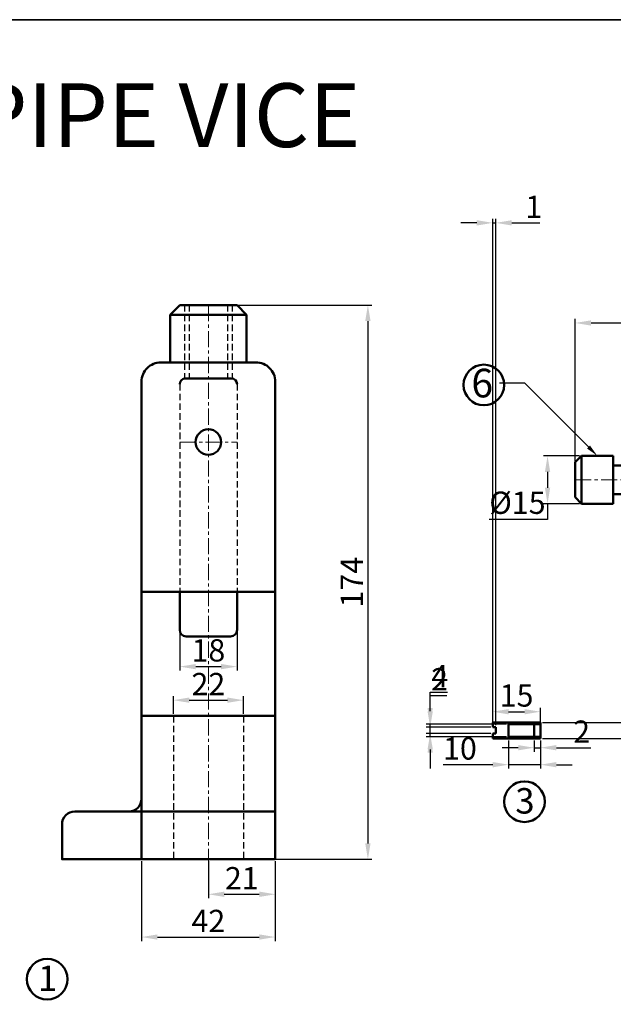
# Model space of a CAD drawing. Units: millimetres. Extents: x -39 to 854, y -107 to 478.
# Tile 3 of 4: x 309 to 496, y 169 to 478. Entities that reach past the tile are written whole.
import ezdxf
from ezdxf import colors
from ezdxf.entities.mleader import LeaderData, LeaderLine
from ezdxf.math import Vec2, Vec3

# ---------------------------------------------------------------- set-up
doc = ezdxf.new("R2010")
doc.units = ezdxf.units.MM
doc.header["$LTSCALE"] = 0.4
doc.linetypes.add('CENTER', pattern=[50.8, 31.75, -6.35, 6.35, -6.35])
doc.linetypes.add('DASHED', pattern=[19.05, 12.7, -6.35])
for name, color, linetype, lineweight in [('M-CNTR', 1, 'CENTER', 18), ('M-DIMS', 2, 'Continuous', 25), ('M-HIDN', 6, 'DASHED', 25), ('M-OUTL', 7, 'Continuous', 50), ('M-TEXT', 3, 'Continuous', 25), ('M-TTLB', 7, 'Continuous', 35)]:
    doc.layers.add(name, color=color, linetype=linetype, lineweight=lineweight)
doc.styles.get("Standard").update_dxf_attribs({"font": 'arial.ttf'})
doc.dimstyles.new('ISO-25', dxfattribs={"dimtxt": 7, "dimasz": 5, "dimexe": 1.25, "dimexo": 0.625, "dimtad": 1, "dimtoh": 1, "dimtxsty": 'Standard', "dimcen": 2.5, "dimadec": 0, "dimazin": 0, "dimtfac": 1, "dimtmove": 0, "dimatfit": 3, "dimfxl": 1, "dimarcsym": 0})

# ---------------------------------------------------------------- blocks, each defined once
blk = doc.blocks.new('*D41')
at = {"layer": 'Defpoints', "color": 0, "ltscale": 0.4, "transparency": 16777216}
for p in [(368.36, 388.19), (368.36, 214.19), (418.49, 214.19)]:
    blk.add_point(p, dxfattribs=at)
at = {"layer": 'M-DIMS', "color": 0, "lineweight": -2, "ltscale": 0.4, "transparency": 16777216}
for p, q in [((368.98, 388.19), (419.74, 388.19)), ((418.49, 383.19), (418.49, 219.19)), ((368.98, 214.19), (419.74, 214.19))]:
    blk.add_line(p, q, dxfattribs=at)
at = {"layer": 'M-DIMS', "color": 0, "ltscale": 0.4, "transparency": 16777216}
for points in [[(417.65, 383.19), (419.32, 383.19), (418.49, 388.19)], [(417.65, 219.19), (419.32, 219.19), (418.49, 214.19)]]:
    blk.add_solid(points, dxfattribs=at)
at = {"layer": 'M-DIMS', "color": 0, "ltscale": 0.4, "transparency": 16777216, "insert": (414.35, 301.19), "char_height": 7, "attachment_point": 5, "rotation": 90}
blk.add_mtext('174', dxfattribs=at)
blk = doc.blocks.new('*D42')
at = {"layer": 'Defpoints', "color": 0, "ltscale": 0.4, "transparency": 16777216}
for p in [(359.36, 292.19), (377.36, 292.19), (377.36, 274.68)]:
    blk.add_point(p, dxfattribs=at)
at = {"layer": 'M-DIMS', "color": 0, "lineweight": -2, "ltscale": 0.4, "transparency": 16777216}
for p, q in [((359.36, 291.56), (359.36, 273.43)), ((377.36, 291.56), (377.36, 273.43)), ((364.36, 274.68), (372.36, 274.68))]:
    blk.add_line(p, q, dxfattribs=at)
at = {"layer": 'M-DIMS', "color": 0, "ltscale": 0.4, "transparency": 16777216}
for points in [[(364.36, 275.51), (364.36, 273.85), (359.36, 274.68)], [(372.36, 275.51), (372.36, 273.85), (377.36, 274.68)]]:
    blk.add_solid(points, dxfattribs=at)
at = {"layer": 'M-DIMS', "color": 0, "ltscale": 0.4, "transparency": 16777216, "insert": (368.36, 278.88), "char_height": 7, "attachment_point": 5}
blk.add_mtext('18', dxfattribs=at)
blk = doc.blocks.new('*D43')
at = {"layer": 'Defpoints', "color": 0, "ltscale": 0.4, "transparency": 16777216}
for p in [(379.36, 264.15), (357.36, 259.19), (379.36, 259.19)]:
    blk.add_point(p, dxfattribs=at)
at = {"layer": 'M-DIMS', "color": 0, "lineweight": -2, "ltscale": 0.4, "transparency": 16777216}
for p, q in [((357.36, 259.81), (357.36, 265.4)), ((362.36, 264.15), (374.36, 264.15)), ((379.36, 259.81), (379.36, 265.4))]:
    blk.add_line(p, q, dxfattribs=at)
at = {"layer": 'M-DIMS', "color": 0, "ltscale": 0.4, "transparency": 16777216}
for points in [[(362.36, 264.98), (362.36, 263.32), (357.36, 264.15)], [(374.36, 264.98), (374.36, 263.32), (379.36, 264.15)]]:
    blk.add_solid(points, dxfattribs=at)
at = {"layer": 'M-DIMS', "color": 0, "ltscale": 0.4, "transparency": 16777216, "insert": (368.36, 268.29), "char_height": 7, "attachment_point": 5}
blk.add_mtext('22', dxfattribs=at)
blk = doc.blocks.new('*D44')
at = {"layer": 'Defpoints', "color": 0, "ltscale": 0.4, "transparency": 16777216}
for p in [(368.36, 214.19), (389.36, 214.19), (389.36, 203.2)]:
    blk.add_point(p, dxfattribs=at)
at = {"layer": 'M-DIMS', "color": 0, "lineweight": -2, "ltscale": 0.4, "transparency": 16777216}
for p, q in [((368.36, 213.56), (368.36, 201.95)), ((389.36, 213.56), (389.36, 201.95)), ((373.36, 203.2), (384.36, 203.2))]:
    blk.add_line(p, q, dxfattribs=at)
at = {"layer": 'M-DIMS', "color": 0, "ltscale": 0.4, "transparency": 16777216}
for points in [[(373.36, 204.03), (373.36, 202.36), (368.36, 203.2)], [(384.36, 204.03), (384.36, 202.36), (389.36, 203.2)]]:
    blk.add_solid(points, dxfattribs=at)
at = {"layer": 'M-DIMS', "color": 0, "ltscale": 0.4, "transparency": 16777216, "insert": (378.86, 207.34), "char_height": 7, "attachment_point": 5}
blk.add_mtext('21', dxfattribs=at)
blk = doc.blocks.new('*D45')
at = {"layer": 'Defpoints', "color": 0, "ltscale": 0.4, "transparency": 16777216}
for p in [(347.36, 214.19), (389.36, 214.19), (389.36, 189.77)]:
    blk.add_point(p, dxfattribs=at)
at = {"layer": 'M-DIMS', "color": 0, "lineweight": -2, "ltscale": 0.4, "transparency": 16777216}
for p, q in [((347.36, 213.56), (347.36, 188.52)), ((389.36, 213.56), (389.36, 188.52)), ((352.36, 189.77), (384.36, 189.77))]:
    blk.add_line(p, q, dxfattribs=at)
at = {"layer": 'M-DIMS', "color": 0, "ltscale": 0.4, "transparency": 16777216}
for points in [[(352.36, 190.6), (352.36, 188.94), (347.36, 189.77)], [(384.36, 190.6), (384.36, 188.94), (389.36, 189.77)]]:
    blk.add_solid(points, dxfattribs=at)
at = {"layer": 'M-DIMS', "color": 0, "ltscale": 0.4, "transparency": 16777216, "insert": (368.36, 193.91), "char_height": 7, "attachment_point": 5}
blk.add_mtext('42', dxfattribs=at)
blk = doc.blocks.new('*D47')
at = {"layer": 'Defpoints', "color": 0, "ltscale": 0.4, "transparency": 16777216}
for p in [(628.63, 382.58), (483.63, 333.34), (628.63, 333.34)]:
    blk.add_point(p, dxfattribs=at)
at = {"layer": 'M-DIMS', "color": 0, "lineweight": -2, "ltscale": 0.4, "transparency": 16777216}
for p, q in [((483.63, 333.96), (483.63, 383.83)), ((628.63, 333.96), (628.63, 383.83)), ((488.63, 382.58), (623.63, 382.58))]:
    blk.add_line(p, q, dxfattribs=at)
at = {"layer": 'M-DIMS', "color": 0, "ltscale": 0.4, "transparency": 16777216}
for points in [[(488.63, 383.41), (488.63, 381.75), (483.63, 382.58)], [(623.63, 383.41), (623.63, 381.75), (628.63, 382.58)]]:
    blk.add_solid(points, dxfattribs=at)
at = {"layer": 'M-DIMS', "color": 0, "ltscale": 0.4, "transparency": 16777216, "insert": (556.13, 386.78), "char_height": 7, "attachment_point": 5}
blk.add_mtext('145', dxfattribs=at)
blk = doc.blocks.new('*D48')
at = {"layer": 'Defpoints', "color": 0, "ltscale": 0.4, "transparency": 16777216}
for p in [(485.63, 340.84), (474.95, 325.84), (485.63, 325.84)]:
    blk.add_point(p, dxfattribs=at)
at = {"layer": 'M-DIMS', "color": 0, "lineweight": -2, "ltscale": 0.4, "transparency": 16777216}
for p, q in [((485, 340.84), (473.7, 340.84)), ((474.95, 335.84), (474.95, 330.84)), ((485, 325.84), (473.7, 325.84)), ((474.95, 325.84), (474.95, 320.84)), ((474.95, 320.84), (456.63, 320.84))]:
    blk.add_line(p, q, dxfattribs=at)
at = {"layer": 'M-DIMS', "color": 0, "ltscale": 0.4, "transparency": 16777216}
for points in [[(474.12, 335.84), (475.79, 335.84), (474.95, 340.84)], [(474.12, 330.84), (475.79, 330.84), (474.95, 325.84)]]:
    blk.add_solid(points, dxfattribs=at)
at = {"layer": 'M-DIMS', "color": 0, "ltscale": 0.4, "transparency": 16777216, "insert": (465.48, 325.23), "char_height": 7, "attachment_point": 5}
blk.add_mtext('%%C15', dxfattribs=at)
blk = doc.blocks.new('*D59')
at = {"layer": 'Defpoints', "color": 0, "ltscale": 0.4, "transparency": 16777216}
for p in [(462.72, 252.16), (472.72, 252.16), (462.72, 243.89)]:
    blk.add_point(p, dxfattribs=at)
at = {"layer": 'M-DIMS', "color": 0, "lineweight": -2, "ltscale": 0.4, "transparency": 16777216}
for p, q in [((462.72, 251.53), (462.72, 242.64)), ((472.72, 251.53), (472.72, 242.64)), ((457.72, 243.89), (442.12, 243.89)), ((472.72, 243.89), (462.72, 243.89)), ((477.72, 243.89), (482.72, 243.89))]:
    blk.add_line(p, q, dxfattribs=at)
at = {"layer": 'M-DIMS', "color": 0, "ltscale": 0.4, "transparency": 16777216}
for points in [[(457.72, 244.72), (457.72, 243.05), (462.72, 243.89)], [(477.72, 244.72), (477.72, 243.05), (472.72, 243.89)]]:
    blk.add_solid(points, dxfattribs=at)
at = {"layer": 'M-DIMS', "color": 0, "ltscale": 0.4, "transparency": 16777216, "insert": (447.42, 248.08), "char_height": 7, "attachment_point": 5}
blk.add_mtext('10', dxfattribs=at)
blk = doc.blocks.new('*D60')
at = {"layer": 'Defpoints', "color": 0, "ltscale": 0.4, "transparency": 16777216}
for p in [(470.72, 252.16), (472.72, 252.16), (472.72, 249.22)]:
    blk.add_point(p, dxfattribs=at)
at = {"layer": 'M-DIMS', "color": 0, "lineweight": -2, "ltscale": 0.4, "transparency": 16777216}
for p, q in [((470.72, 251.53), (470.72, 247.97)), ((472.72, 251.53), (472.72, 247.97)), ((465.72, 249.22), (460.72, 249.22)), ((470.72, 249.22), (472.72, 249.22)), ((477.72, 249.22), (488.6, 249.22))]:
    blk.add_line(p, q, dxfattribs=at)
at = {"layer": 'M-DIMS', "color": 0, "ltscale": 0.4, "transparency": 16777216}
for points in [[(465.72, 250.05), (465.72, 248.38), (470.72, 249.22)], [(477.72, 250.05), (477.72, 248.38), (472.72, 249.22)]]:
    blk.add_solid(points, dxfattribs=at)
at = {"layer": 'M-DIMS', "color": 0, "ltscale": 0.4, "transparency": 16777216, "insert": (485.66, 253.36), "char_height": 7, "attachment_point": 5}
blk.add_mtext('2', dxfattribs=at)
blk = doc.blocks.new('*D61')
at = {"layer": 'Defpoints', "color": 0, "ltscale": 0.4, "transparency": 16777216}
for p in [(472.72, 260.52), (457.72, 257.16), (472.72, 256.66)]:
    blk.add_point(p, dxfattribs=at)
at = {"layer": 'M-DIMS', "color": 0, "lineweight": -2, "ltscale": 0.4, "transparency": 16777216}
for p, q in [((457.72, 257.78), (457.72, 261.77)), ((462.72, 260.52), (467.72, 260.52)), ((472.72, 257.28), (472.72, 261.77))]:
    blk.add_line(p, q, dxfattribs=at)
at = {"layer": 'M-DIMS', "color": 0, "ltscale": 0.4, "transparency": 16777216}
for points in [[(462.72, 261.35), (462.72, 259.69), (457.72, 260.52)], [(467.72, 261.35), (467.72, 259.69), (472.72, 260.52)]]:
    blk.add_solid(points, dxfattribs=at)
at = {"layer": 'M-DIMS', "color": 0, "ltscale": 0.4, "transparency": 16777216, "insert": (465.22, 264.72), "char_height": 7, "attachment_point": 5}
blk.add_mtext('15', dxfattribs=at)
blk = doc.blocks.new('HANDLE-BAR')
at = {"ltscale": 0.4}
for p, q in [((48.5, 20), (50.5, 22)), ((50.5, 22), (70.5, 22)), ((70.5, 22), (72.5, 20)), ((48.5, 20), (72.5, 20)), ((48.5, 14.5), (48.5, 20)), ((72.5, 20), (72.5, 14.5)), ((48.5, 14.5), (0, 14.5)), ((72.5, 14.5), (121, 14.5)), ((48.5, 5.5), (0, 5.5)), ((48.5, 0), (48.5, 5.5)), ((72.5, 5.5), (121, 5.5)), ((72.5, 5.5), (72.5, 0)), ((72.5, 0), (48.5, 0))]:
    blk.add_line(p, q, dxfattribs=at)
for centre, start, end in [((44.46, 10), 311.9139, 48.0861), ((76.54, 10), 131.9139, 228.0861)]:
    blk.add_arc(centre, 6.05, start, end, dxfattribs=at)
blk = doc.blocks.new('HANDLE-BAR-CAP')
at = {"ltscale": 0.4}
for p, q in [((10, 15), (0, 15)), ((0, 15), (0, 0)), ((12, 13), (10, 15)), ((10, 15), (10, 0)), ((12, 2), (12, 13)), ((0, 0), (10, 0)), ((12, 2), (10, 0))]:
    blk.add_line(p, q, dxfattribs=at)
blk = doc.blocks.new('*D75')
at = {"layer": 'Defpoints', "color": 0, "ltscale": 0.4, "transparency": 16777216}
for p in [(472.72, 257.16), (639.13, 257.16), (472.72, 252.16)]:
    blk.add_point(p, dxfattribs=at)
at = {"layer": 'M-DIMS', "color": 0, "lineweight": -2, "ltscale": 0.4, "transparency": 16777216}
for p, q in [((639.13, 262.16), (639.13, 267.16)), ((639.13, 267.16), (644.39, 267.16)), ((473.34, 257.16), (640.38, 257.16)), ((639.13, 252.16), (639.13, 257.16)), ((473.34, 252.16), (640.38, 252.16)), ((639.13, 247.16), (639.13, 242.16))]:
    blk.add_line(p, q, dxfattribs=at)
at = {"layer": 'M-DIMS', "color": 0, "ltscale": 0.4, "transparency": 16777216}
for points in [[(638.29, 262.16), (639.96, 262.16), (639.13, 257.16)], [(638.29, 247.16), (639.96, 247.16), (639.13, 252.16)]]:
    blk.add_solid(points, dxfattribs=at)
at = {"layer": 'M-DIMS', "color": 0, "ltscale": 0.4, "transparency": 16777216, "insert": (642.07, 271.34), "char_height": 7, "attachment_point": 5}
blk.add_mtext('5', dxfattribs=at)
blk = doc.blocks.new('*D76')
at = {"layer": 'Defpoints', "color": 0, "ltscale": 0.4, "transparency": 16777216}
for p in [(438.06, 256.66), (462.72, 256.66), (462.72, 252.66)]:
    blk.add_point(p, dxfattribs=at)
at = {"layer": 'M-DIMS', "color": 0, "lineweight": -2, "ltscale": 0.4, "transparency": 16777216}
for p, q in [((438.06, 261.66), (438.06, 266.66)), ((438.06, 266.66), (443.53, 266.66)), ((462.09, 256.66), (436.81, 256.66)), ((438.06, 252.66), (438.06, 256.66)), ((462.09, 252.66), (436.81, 252.66)), ((438.06, 247.66), (438.06, 242.66))]:
    blk.add_line(p, q, dxfattribs=at)
at = {"layer": 'M-DIMS', "color": 0, "ltscale": 0.4, "transparency": 16777216}
for points in [[(437.23, 261.66), (438.9, 261.66), (438.06, 256.66)], [(437.23, 247.66), (438.9, 247.66), (438.06, 252.66)]]:
    blk.add_solid(points, dxfattribs=at)
at = {"layer": 'M-DIMS', "color": 0, "ltscale": 0.4, "transparency": 16777216, "insert": (441.11, 270.78), "char_height": 7, "attachment_point": 5}
blk.add_mtext('4', dxfattribs=at)
blk = doc.blocks.new('*D77')
at = {"layer": 'Defpoints', "color": 0, "ltscale": 0.4, "transparency": 16777216}
for p in [(438.06, 255.66), (457.72, 255.66), (457.72, 253.66)]:
    blk.add_point(p, dxfattribs=at)
at = {"layer": 'M-DIMS', "color": 0, "lineweight": -2, "ltscale": 0.4, "transparency": 16777216}
for p, q in [((438.06, 260.66), (438.06, 265.66)), ((438.06, 265.66), (443.33, 265.66)), ((457.09, 255.66), (436.81, 255.66)), ((457.09, 253.66), (436.81, 253.66)), ((438.06, 253.66), (438.06, 255.66)), ((438.06, 248.66), (438.06, 243.66))]:
    blk.add_line(p, q, dxfattribs=at)
at = {"layer": 'M-DIMS', "color": 0, "ltscale": 0.4, "transparency": 16777216}
for points in [[(437.23, 260.66), (438.9, 260.66), (438.06, 255.66)], [(437.23, 248.66), (438.9, 248.66), (438.06, 253.66)]]:
    blk.add_solid(points, dxfattribs=at)
at = {"layer": 'M-DIMS', "color": 0, "ltscale": 0.4, "transparency": 16777216, "insert": (441.01, 269.8), "char_height": 7, "attachment_point": 5}
blk.add_mtext('2', dxfattribs=at)
blk = doc.blocks.new('*D78')
at = {"layer": 'Defpoints', "color": 0, "ltscale": 0.4, "transparency": 16777216}
for p in [(458.72, 414.02), (457.72, 255.66), (458.72, 255.66)]:
    blk.add_point(p, dxfattribs=at)
at = {"layer": 'M-DIMS', "color": 0, "lineweight": -2, "ltscale": 0.4, "transparency": 16777216}
for p, q in [((457.72, 256.28), (457.72, 415.27)), ((458.72, 256.28), (458.72, 415.27)), ((452.72, 414.02), (447.72, 414.02)), ((457.72, 414.02), (458.72, 414.02)), ((463.72, 414.02), (472.55, 414.02))]:
    blk.add_line(p, q, dxfattribs=at)
at = {"layer": 'M-DIMS', "color": 0, "ltscale": 0.4, "transparency": 16777216}
for points in [[(452.72, 414.85), (452.72, 413.18), (457.72, 414.02)], [(463.72, 414.85), (463.72, 413.18), (458.72, 414.02)]]:
    blk.add_solid(points, dxfattribs=at)
at = {"layer": 'M-DIMS', "color": 0, "ltscale": 0.4, "transparency": 16777216, "insert": (470.63, 418.15), "char_height": 7, "attachment_point": 5}
blk.add_mtext('1', dxfattribs=at)

msp = doc.modelspace()

# ---------------------------------------------------------------- linework, layer by layer
at = {"layer": 'M-CNTR', "ltscale": 0.4}
for p, q in [((368.355, 388.187), (368.355, 201.704)), ((359.355, 345.187), (377.355, 345.187)), ((483.627, 333.335), (628.627, 333.335))]:
    msp.add_line(p, q, dxfattribs=at)
at = {"layer": 'M-HIDN', "ltscale": 0.4}
for p, q in [((360.855, 388.187), (360.855, 365.162)), ((362.355, 388.187), (362.355, 365.187)), ((374.355, 388.187), (374.355, 365.187)), ((375.855, 388.187), (375.855, 365.162)), ((359.355, 363.387), (359.355, 298.187)), ((377.355, 363.387), (377.355, 298.187)), ((357.355, 259.187), (357.355, 214.187)), ((379.355, 259.187), (379.355, 214.187))]:
    msp.add_line(p, q, dxfattribs=at)
at = {"layer": 'M-OUTL', "ltscale": 0.4}
for p, q in [((359.355, 388.187), (356.355, 385.187)), ((377.355, 388.187), (359.355, 388.187)), ((377.355, 388.187), (380.355, 385.187)), ((356.355, 385.187), (356.355, 370.187)), ((356.355, 385.187), (380.355, 385.187)), ((380.355, 385.187), (380.355, 370.187)), ((361.155, 365.187), (375.555, 365.187)), ((389.355, 298.187), (347.355, 298.187)), ((359.355, 298.187), (359.355, 286.187)), ((377.355, 298.187), (377.355, 286.187)), ((361.355, 284.187), (375.355, 284.187)), ((347.355, 259.187), (389.355, 259.187)), ((457.718, 257.157), (472.718, 257.157)), ((457.718, 255.657), (457.718, 257.157)), ((462.718, 252.157), (462.718, 257.157)), ((462.718, 256.657), (472.718, 256.657)), ((470.718, 257.157), (470.718, 252.157)), ((472.718, 257.157), (472.718, 252.157)), ((458.718, 255.657), (457.718, 255.657)), ((457.718, 252.157), (457.718, 253.657)), ((458.718, 253.657), (457.718, 253.657)), ((458.718, 254.657), (458.718, 255.657)), ((458.718, 254.657), (458.718, 253.657)), ((472.718, 252.157), (457.718, 252.157)), ((472.718, 252.657), (462.718, 252.657)), ((347.355, 233.187), (347.355, 214.187)), ((347.355, 214.187), (389.355, 214.187))]:
    msp.add_line(p, q, dxfattribs=at)
msp.add_lwpolyline([(347.355, 214.187), (322.355, 214.187), (322.355, 225.187, -0.4142136), (326.355, 229.187), (332.355, 229.187), (343.355, 229.187, 0.4142136), (347.355, 233.187), (347.355, 364.187, -0.4142136), (353.355, 370.187), (383.355, 370.187, -0.4142136), (389.355, 364.187), (389.355, 214.187)], format="xyb", dxfattribs=at)
msp.add_lwpolyline([(343.355, 229.187), (389.355, 229.187)], dxfattribs=at)
for centre, radius in [((454.946, 363.119), 6.382), ((368.355, 345.187), 4), ((467.703, 232.262), 6.382), ((317.703, 176.545), 6.382)]:
    msp.add_circle(centre, radius, dxfattribs=at)
for centre, radius, start, end in [((361.155, 363.387), 1.8, 90, 180), ((375.555, 363.387), 1.8, 360, 90), ((361.355, 286.187), 2, 180, 270), ((375.355, 286.187), 2, 270, 0)]:
    msp.add_arc(centre, radius, start, end, dxfattribs=at)
at = {"layer": 'M-TTLB', "ltscale": 0.4}
msp.add_lwpolyline([(-38.928, 477.809), (854.289, 477.809), (854.289, -107.035), (-38.928, -107.035)], close=True, dxfattribs=at)

# ---------------------------------------------------------------- block references
at = {"layer": 'M-OUTL'}
msp.add_blockref('HANDLE-BAR', (495.627, 323.335), dxfattribs=at)
at = {"layer": 'M-OUTL', "rotation": 180}
msp.add_blockref('HANDLE-BAR-CAP', (495.627, 340.836), dxfattribs=at)

# ---------------------------------------------------------------- texts
at = {"layer": 'M-TEXT', "ltscale": 0.4, "attachment_point": 1}
for s, width, insert, char_height in [('PIPE VICE', 220.27302, (294.238, 457.823), 20), ('3', 4.03665, (464.811, 236.536), 8), ('1', 4.03665, (314.811, 180.819), 8)]:
    msp.add_mtext_dynamic_manual_height_columns(s, width=width, gutter_width=12.5, heights=[0], dxfattribs=dict(at, insert=insert, char_height=char_height))

# ---------------------------------------------------------------- dimensions: what is measured, and where the dimension line sits
at = {"layer": 'M-DIMS', "ltscale": 0.4}
for base, p1, p2, override, picture, middle in [((458.718, 414.015), (457.718, 255.657), (458.718, 255.657), {"dimdec": 0, "dimlfac": 1, "dimrnd": 0, "dimzin": 0, "dimdsep": 46, "dimlunit": 2}, '*D78', (470.632, 418.155)), ((628.627, 382.578), (483.627, 333.335), (628.627, 333.335), {"dimclrd": 0, "dimclre": 0, "dimclrt": 0}, '*D47', (556.127, 386.777)), ((377.355, 274.681), (359.355, 292.187), (377.355, 292.187), {"dimclrd": 0, "dimclre": 0, "dimclrt": 0}, '*D42', (368.355, 278.88)), ((379.355, 264.15), (357.355, 259.187), (379.355, 259.187), {"dimclrd": 0, "dimclre": 0, "dimclrt": 0}, '*D43', (368.355, 268.289)), ((472.718, 260.52), (457.718, 257.157), (472.718, 256.657), {"dimclrd": 0, "dimclre": 0, "dimclrt": 0}, '*D61', (465.218, 264.719)), ((472.718, 249.218), (470.718, 252.157), (472.718, 252.157), {"dimclrd": 0, "dimclre": 0, "dimclrt": 0}, '*D60', (485.661, 253.357)), ((462.718, 243.885), (472.718, 252.157), (462.718, 252.157), {"dimclrd": 0, "dimclre": 0, "dimclrt": 0}, '*D59', (447.42, 248.084)), ((389.355, 189.769), (347.355, 214.187), (389.355, 214.187), {"dimclrd": 0, "dimclre": 0, "dimclrt": 0}, '*D45', (368.355, 193.908)), ((389.355, 203.198), (368.355, 214.187), (389.355, 214.187), {"dimclrd": 0, "dimclre": 0, "dimclrt": 0}, '*D44', (378.855, 207.338))]:
    dim = msp.add_linear_dim(base=base, p1=p1, p2=p2, dimstyle='ISO-25', override=override, dxfattribs=at)
    dim.commit()
    dim.dimension.update_dxf_attribs({"geometry": picture, "text_midpoint": middle})
for base, p1, p2, override, picture, middle in [((418.485, 214.187), (368.355, 388.187), (368.355, 214.187), {"dimclrd": 0, "dimclre": 0, "dimclrt": 0}, '*D41', (414.346, 301.187)), ((438.064, 256.657), (462.718, 252.657), (462.718, 256.657), {"dimdec": 0, "dimlfac": 1, "dimrnd": 0, "dimzin": 0, "dimdsep": 46, "dimlunit": 2}, '*D76', (441.11, 270.782)), ((639.127, 257.157), (472.718, 252.157), (472.718, 257.157), {"dimdec": 0, "dimlfac": 1, "dimrnd": 0, "dimzin": 0, "dimdsep": 46, "dimlunit": 2}, '*D75', (642.072, 271.341)), ((438.064, 255.657), (457.718, 253.657), (457.718, 255.657), {"dimdec": 0, "dimlfac": 1, "dimrnd": 0, "dimzin": 0, "dimdsep": 46, "dimlunit": 2}, '*D77', (441.007, 269.796))]:
    dim = msp.add_linear_dim(base=base, p1=p1, p2=p2, angle=90, dimstyle='ISO-25', override=override, dxfattribs=at)
    dim.commit()
    dim.dimension.update_dxf_attribs({"geometry": picture, "text_midpoint": middle})
dim = msp.add_linear_dim(base=(474.953, 325.835), p1=(485.627, 340.835), p2=(485.627, 325.835), angle=90, text='%%C<>', dimstyle='ISO-25', override={"dimclrd": 0, "dimclre": 0, "dimclrt": 0}, dxfattribs=at)
dim.commit()
dim.dimension.update_dxf_attribs({"geometry": '*D48', "text_midpoint": (465.48, 325.23)})

# ---------------------------------------------------------------- leaders
at = {"layer": 'M-TEXT', "ltscale": 0.4}
ml = msp.add_multileader_mtext('Standard', dxfattribs=at)
ml.set_content('6', color=256)
ml.set_leader_properties()
ml.build(insert=Vec2(0, 0))
ctx = ml.context
ctx.base_point, ctx.char_height, ctx.plane_origin = Vec3(449.882, 363.637), 9, Vec3(490.627, 340.835)
ctx.text_align_type = 2
notes = []
notes.append((ctx, [(0, (1, 1, 0), (467.825, 363.637), (-1, 0), 8, [(0, [(490.627, 340.835)], 0, [])])]))
ctx.mtext.insert, ctx.mtext.alignment, ctx.mtext.flow_direction = Vec3(457.825, 368.214), 3, 5
for ctx, leaders in notes:
    for number, flags, end, landing, length, lines in leaders:
        leader = LeaderData()
        leader.index, (leader.has_last_leader_line, leader.has_dogleg_vector, leader.attachment_direction) = number, flags
        leader.last_leader_point, leader.dogleg_vector, leader.dogleg_length = Vec3(end), Vec3(landing), length
        for number, points, colour, breaks in lines:
            line = LeaderLine()
            line.index, line.vertices, line.color, line.breaks = number, Vec3.list(points), colors.encode_raw_color(colour), breaks
            leader.lines.append(line)
        ctx.leaders.append(leader)

doc.saveas('drawing.dxf')
